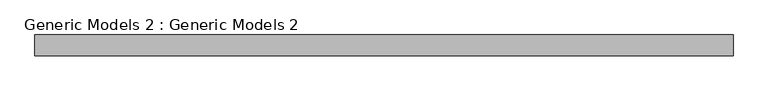
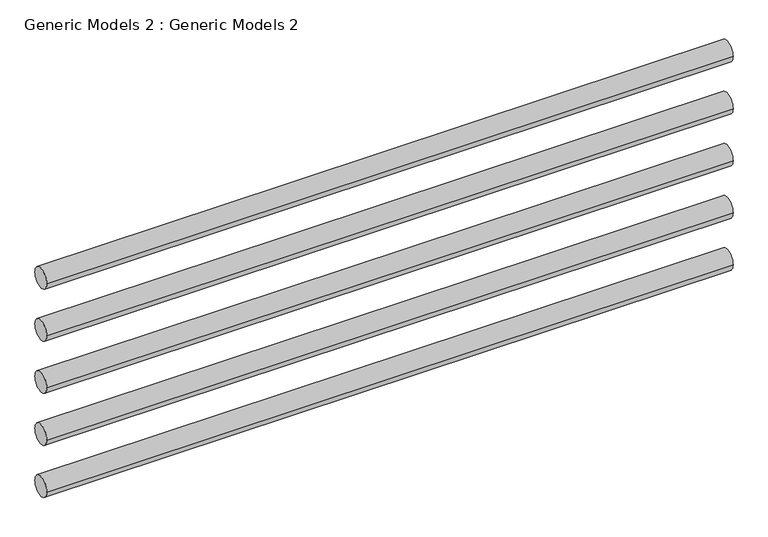
"""IFC4 building model written with IfcOpenShell, lengths in millimetres: proxy geometry, Generic Models 2 : Generic Models 2."""

from ifc_helpers import new_model, si_unit, point, frame, frame_2d, origin, place, context, project, spatial, circle_curve, trimmed, segment, composite_curve, outline, extrude, source, transform, mapped, element, save


def generic_models_2_generic_models_2_a69240e3(model_context):
    return source(origin(), model_context, "Body", "SweptSolid", [
        extrude(outline(composite_curve([segment(trimmed(circle_curve(frame_2d((-4381.7724035, 7808.1544804)), 38.1), [point((-4419.8724035, 7808.1544804))], [point((-4343.6724035, 7808.1544804))], False, "CARTESIAN"), True, "CONTINUOUS"), segment(trimmed(circle_curve(frame_2d((-4381.7724035, 7808.1544804)), 38.1), [point((-4343.6724035, 7808.1544804))], [point((-4419.8724035, 7808.1544804))], False, "CARTESIAN"), True, "CONTINUOUS")], self_intersect=False)), frame((-14722.761259, 0.0, 0.0), z_axis=(1.0, 0.0, 0.0), x_axis=(0.0, 1.0, 0.0)), (0.0, 0.0, 1.0), 2531.6821699),
        extrude(outline(composite_curve([segment(trimmed(circle_curve(frame_2d((-4381.7724035, 7604.9544804)), 38.1), [point((-4419.8724035, 7604.9544804))], [point((-4343.6724035, 7604.9544804))], False, "CARTESIAN"), True, "CONTINUOUS"), segment(trimmed(circle_curve(frame_2d((-4381.7724035, 7604.9544804)), 38.1), [point((-4343.6724035, 7604.9544804))], [point((-4419.8724035, 7604.9544804))], False, "CARTESIAN"), True, "CONTINUOUS")], self_intersect=False)), frame((-14722.761259, 0.0, 0.0), z_axis=(1.0, 0.0, 0.0), x_axis=(0.0, 1.0, 0.0)), (0.0, 0.0, 1.0), 2531.6821699),
        extrude(outline(composite_curve([segment(trimmed(circle_curve(frame_2d((-4381.7724035, 7401.7544804)), 38.1), [point((-4419.8724035, 7401.7544804))], [point((-4343.6724035, 7401.7544804))], False, "CARTESIAN"), True, "CONTINUOUS"), segment(trimmed(circle_curve(frame_2d((-4381.7724035, 7401.7544804)), 38.1), [point((-4343.6724035, 7401.7544804))], [point((-4419.8724035, 7401.7544804))], False, "CARTESIAN"), True, "CONTINUOUS")], self_intersect=False)), frame((-14722.761259, 0.0, 0.0), z_axis=(1.0, 0.0, 0.0), x_axis=(0.0, 1.0, 0.0)), (0.0, 0.0, 1.0), 2531.6821699),
        extrude(outline(composite_curve([segment(trimmed(circle_curve(frame_2d((-4381.7724035, 7198.5544804)), 38.1), [point((-4419.8724035, 7198.5544804))], [point((-4343.6724035, 7198.5544804))], False, "CARTESIAN"), True, "CONTINUOUS"), segment(trimmed(circle_curve(frame_2d((-4381.7724035, 7198.5544804)), 38.1), [point((-4343.6724035, 7198.5544804))], [point((-4419.8724035, 7198.5544804))], False, "CARTESIAN"), True, "CONTINUOUS")], self_intersect=False)), frame((-14722.761259, 0.0, 0.0), z_axis=(1.0, 0.0, 0.0), x_axis=(0.0, 1.0, 0.0)), (0.0, 0.0, 1.0), 2531.6821699),
        extrude(outline(composite_curve([segment(trimmed(circle_curve(frame_2d((-4381.7724035, 6995.3544804)), 38.1), [point((-4419.8724035, 6995.3544804))], [point((-4343.6724035, 6995.3544804))], False, "CARTESIAN"), True, "CONTINUOUS"), segment(trimmed(circle_curve(frame_2d((-4381.7724035, 6995.3544804)), 38.1), [point((-4343.6724035, 6995.3544804))], [point((-4419.8724035, 6995.3544804))], False, "CARTESIAN"), True, "CONTINUOUS")], self_intersect=False)), frame((-14722.761259, 0.0, 0.0), z_axis=(1.0, 0.0, 0.0), x_axis=(0.0, 1.0, 0.0)), (0.0, 0.0, 1.0), 2531.6821699),
    ])


if __name__ == "__main__":
    model = new_model("IFC4")
    model_context = context("Model", 3, world=origin())
    ifc_project = project(units=[si_unit("LENGTHUNIT", "METRE", prefix="MILLI")], contexts=[model_context])
    site = spatial("IfcSite", under=ifc_project)
    building = spatial("IfcBuilding", under=site)
    placement = place(None, origin())
    generic_models_2_generic_models_2_shape = generic_models_2_generic_models_2_a69240e3(model_context)
    element("IfcBuildingElementProxy", 1, Name="Generic Models 2 : Generic Models 2", ObjectType="Generic Models 2 : Generic Models 2", at=placement, inside=building, context=model_context, shape_type="MappedRepresentation", body=[
        mapped(generic_models_2_generic_models_2_shape, transform((0.0, 0.0, 0.0), x_axis=(1.0, 0.0, 0.0), y_axis=(0.0, 1.0, 0.0), z_axis=(0.0, 0.0, 1.0))),
    ])
    save(model, "model.ifc")
